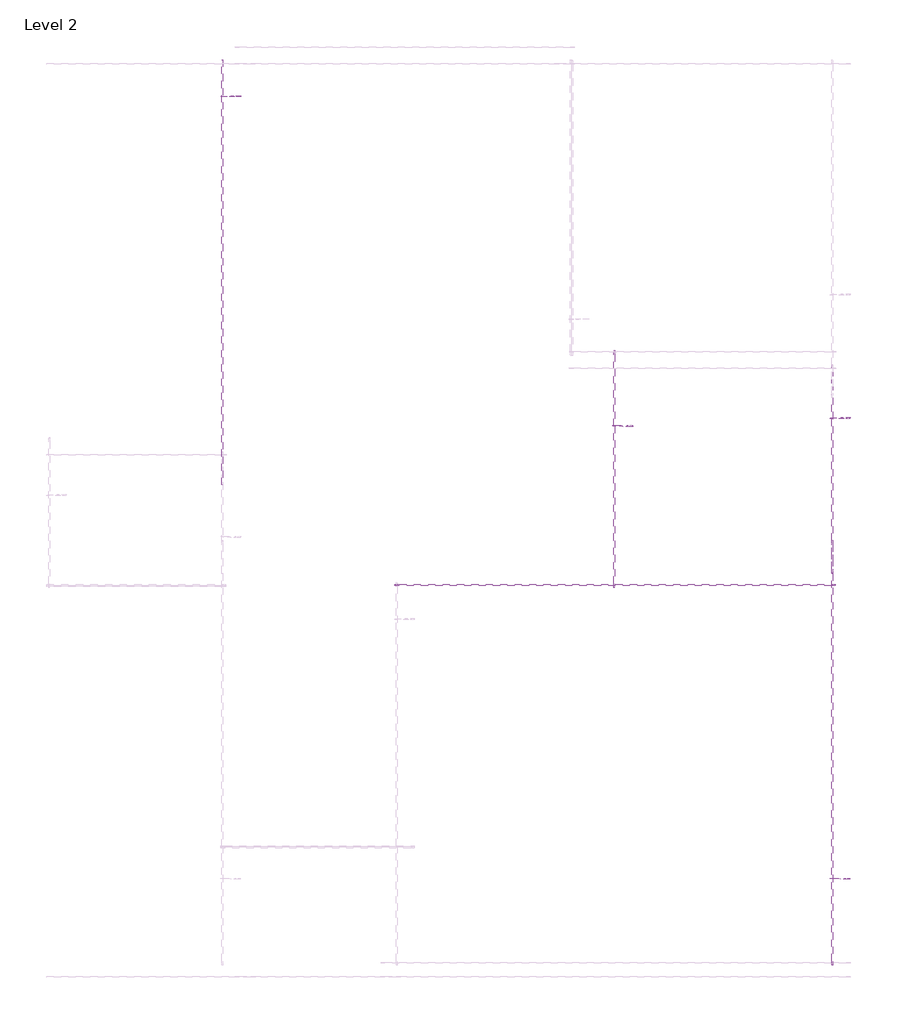
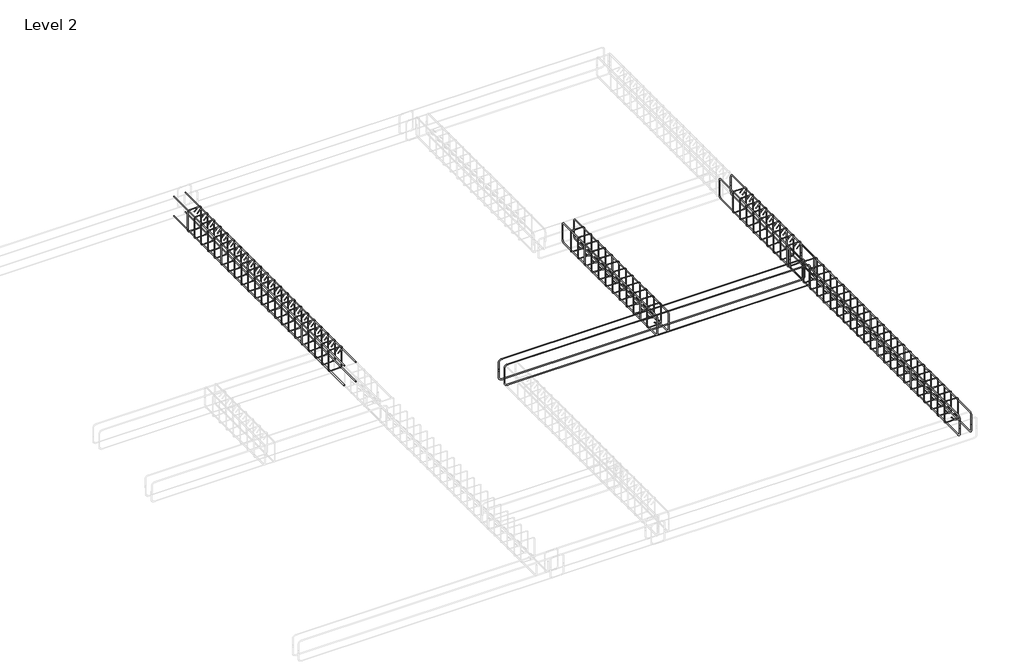
# One storey, part 4 of 5: 14 reinforcing bars.
"""IFC4 building model written with IfcOpenShell, lengths in millimetres."""

from ifc_helpers import new_model, si_unit, point, frame, origin, place, context, project, spatial, polyline, circle_curve, trimmed, segment, composite_curve, source, transform, mapped, element, save
from ifc_brep_helpers import swept_disk

model = new_model("IFC4")

# Units and contexts
model_context = context("Model", 3, world=origin())
ifc_project = project(units=[si_unit("LENGTHUNIT", "METRE", prefix="MILLI")], contexts=[model_context])

# Site, building, storey
site = spatial("IfcSite", under=ifc_project)
building = spatial("IfcBuilding", under=site)
storey = spatial("IfcBuildingStorey", under=building, Name="Level 2", Elevation=3048.0)

# Reinforcing bars
placement = place(None, origin())
reinforcing_bar_shape = source(origin(), model_context, "Body", "SolidModel", [
    swept_disk(composite_curve([segment(polyline([(-4212.455746, 4821.0577522, 5841.8967919), (-4212.455746, 4821.0577522, 5994.2967919)]), True, "CONTINUOUS"), segment(trimmed(circle_curve(frame((-4212.455746, 4776.9887522, 5994.2967919), z_axis=(1.0, 0.0, 0.0), x_axis=(0.0, 44.069000000000415, 0.0)), 44.069), [point((-4212.455746, 4821.0577522, 5994.2967919))], [point((-4212.455746, 4776.9887522, 6038.3657919))], True, "CARTESIAN"), True, "CONTINUOUS"), segment(polyline([(-4212.455746, 4776.9887522, 6038.3657919), (-4212.455746, 2478.6647522, 6038.3657919)]), True, "CONTINUOUS"), segment(trimmed(circle_curve(frame((-4212.455746, 2478.6647522, 5994.2967919), z_axis=(1.0, 0.0, 0.0), x_axis=(0.0, 0.0, 44.068999999999505)), 44.069), [point((-4212.455746, 2478.6647522, 6038.3657919))], [point((-4212.455746, 2434.5957522, 5994.2967919))], True, "CARTESIAN"), True, "CONTINUOUS"), segment(polyline([(-4212.455746, 2434.5957522, 5994.2967919), (-4212.455746, 2434.5957522, 5841.8967919)]), True, "CONTINUOUS")], self_intersect=False), 5.969),
])
element("IfcReinforcingBar", 1, at=placement, inside=storey, context=model_context, shape_type="MappedRepresentation", body=[
    mapped(reinforcing_bar_shape, transform((0.0, 0.0, 0.0), x_axis=(1.0, 0.0, 0.0), y_axis=(0.0, 1.0, 0.0), z_axis=(0.0, 0.0, 1.0))),
    mapped(reinforcing_bar_shape, transform((-189.5315837, 0.0, 0.0), x_axis=(1.0, 0.0, 0.0), y_axis=(0.0, 1.0, 0.0), z_axis=(0.0, 0.0, 1.0))),
])
reinforcing_bar_2_shape = source(origin(), model_context, "Body", "SolidModel", [
    swept_disk(composite_curve([segment(polyline([(-4212.455746, 2434.5957522, 5892.9032081), (-4212.455746, 2434.5957522, 5740.5032081)]), True, "CONTINUOUS"), segment(trimmed(circle_curve(frame((-4212.455746, 2478.6647522, 5740.5032081), z_axis=(1.0, 0.0, 0.0), x_axis=(0.0, -44.06899999999996, 0.0)), 44.069), [point((-4212.455746, 2434.5957522, 5740.5032081))], [point((-4212.455746, 2478.6647522, 5696.4342081))], True, "CARTESIAN"), True, "CONTINUOUS"), segment(polyline([(-4212.455746, 2478.6647522, 5696.4342081), (-4212.455746, 4776.9887522, 5696.4342081)]), True, "CONTINUOUS"), segment(trimmed(circle_curve(frame((-4212.455746, 4776.9887522, 5740.5032081), z_axis=(1.0, 0.0, 0.0), x_axis=(0.0, 0.0, -44.068999999999505)), 44.069), [point((-4212.455746, 4776.9887522, 5696.4342081))], [point((-4212.455746, 4821.0577522, 5740.5032081))], True, "CARTESIAN"), True, "CONTINUOUS"), segment(polyline([(-4212.455746, 4821.0577522, 5740.5032081), (-4212.455746, 4821.0577522, 5892.9032081)]), True, "CONTINUOUS")], self_intersect=False), 5.969),
])
element("IfcReinforcingBar", 2, at=placement, inside=storey, context=model_context, shape_type="MappedRepresentation", body=[
    mapped(reinforcing_bar_2_shape, transform((0.0, 0.0, 0.0), x_axis=(1.0, 0.0, 0.0), y_axis=(0.0, 1.0, 0.0), z_axis=(0.0, 0.0, 1.0))),
    mapped(reinforcing_bar_2_shape, transform((-189.5315837, 0.0, 0.0), x_axis=(1.0, 0.0, 0.0), y_axis=(0.0, 1.0, 0.0), z_axis=(0.0, 0.0, 1.0))),
])
reinforcing_bar_3_shape = source(origin(), model_context, "Body", "SolidModel", [
    swept_disk(composite_curve([segment(polyline([(-4212.455746, 2803.6577522, 5841.8967919), (-4212.455746, 2803.6577522, 5994.2967919)]), True, "CONTINUOUS"), segment(trimmed(circle_curve(frame((-4212.455746, 2759.5887522, 5994.2967919), z_axis=(1.0, 0.0, 0.0), x_axis=(0.0, 44.06899999999996, 0.0)), 44.069), [point((-4212.455746, 2803.6577522, 5994.2967919))], [point((-4212.455746, 2759.5887522, 6038.3657919))], True, "CARTESIAN"), True, "CONTINUOUS"), segment(polyline([(-4212.455746, 2759.5887522, 6038.3657919), (-4212.455746, -2021.3352478, 6038.3657919)]), True, "CONTINUOUS"), segment(trimmed(circle_curve(frame((-4212.455746, -2021.3352478, 5994.2967919), z_axis=(1.0, 0.0, 0.0), x_axis=(0.0, 0.0, 44.068999999999505)), 44.069), [point((-4212.455746, -2021.3352478, 6038.3657919))], [point((-4212.455746, -2065.4042478, 5994.2967919))], True, "CARTESIAN"), True, "CONTINUOUS"), segment(polyline([(-4212.455746, -2065.4042478, 5994.2967919), (-4212.455746, -2065.4042478, 5841.8967919)]), True, "CONTINUOUS")], self_intersect=False), 5.969),
])
element("IfcReinforcingBar", 3, at=placement, inside=storey, context=model_context, shape_type="MappedRepresentation", body=[
    mapped(reinforcing_bar_3_shape, transform((0.0, 0.0, 0.0), x_axis=(1.0, 0.0, 0.0), y_axis=(0.0, 1.0, 0.0), z_axis=(0.0, 0.0, 1.0))),
    mapped(reinforcing_bar_3_shape, transform((-189.5315837, 0.0, 0.0), x_axis=(1.0, 0.0, 0.0), y_axis=(0.0, 1.0, 0.0), z_axis=(0.0, 0.0, 1.0))),
])
reinforcing_bar_4_shape = source(origin(), model_context, "Body", "SolidModel", [
    swept_disk(composite_curve([segment(polyline([(-4212.455746, -2065.4042478, 5892.9032081), (-4212.455746, -2065.4042478, 5740.5032081)]), True, "CONTINUOUS"), segment(trimmed(circle_curve(frame((-4212.455746, -2021.3352478, 5740.5032081), z_axis=(1.0, 0.0, 0.0), x_axis=(0.0, -44.06900000000019, 0.0)), 44.069), [point((-4212.455746, -2065.4042478, 5740.5032081))], [point((-4212.455746, -2021.3352478, 5696.4342081))], True, "CARTESIAN"), True, "CONTINUOUS"), segment(polyline([(-4212.455746, -2021.3352478, 5696.4342081), (-4212.455746, 2759.5887522, 5696.4342081)]), True, "CONTINUOUS"), segment(trimmed(circle_curve(frame((-4212.455746, 2759.5887522, 5740.5032081), z_axis=(1.0, 0.0, 0.0), x_axis=(0.0, 0.0, -44.068999999999505)), 44.069), [point((-4212.455746, 2759.5887522, 5696.4342081))], [point((-4212.455746, 2803.6577522, 5740.5032081))], True, "CARTESIAN"), True, "CONTINUOUS"), segment(polyline([(-4212.455746, 2803.6577522, 5740.5032081), (-4212.455746, 2803.6577522, 5892.9032081)]), True, "CONTINUOUS")], self_intersect=False), 5.969),
])
element("IfcReinforcingBar", 4, at=placement, inside=storey, context=model_context, shape_type="MappedRepresentation", body=[
    mapped(reinforcing_bar_4_shape, transform((0.0, 0.0, 0.0), x_axis=(1.0, 0.0, 0.0), y_axis=(0.0, 1.0, 0.0), z_axis=(0.0, 0.0, 1.0))),
    mapped(reinforcing_bar_4_shape, transform((-189.5315837, 0.0, 0.0), x_axis=(1.0, 0.0, 0.0), y_axis=(0.0, 1.0, 0.0), z_axis=(0.0, 0.0, 1.0))),
])
reinforcing_bar_5_shape = source(origin(), model_context, "Body", "SolidModel", [
    swept_disk(composite_curve([segment(polyline([(-4260.3161447, -1648.3362478, 5785.7833901), (-4205.4511463, -1648.3362478, 5730.9183916)]), True, "CONTINUOUS"), segment(trimmed(circle_curve(frame((-4226.1955379, -1648.3362478, 5710.174), z_axis=(0.0, 1.0, 0.0), x_axis=(20.7443916000002, 0.0, 20.7443916000002)), 29.337), [point((-4205.4511463, -1648.3362478, 5730.9183916))], [point((-4226.1955379, -1648.3362478, 5680.837))], True, "CARTESIAN"), True, "CONTINUOUS"), segment(polyline([(-4226.1955379, -1648.3362478, 5680.837), (-4388.2475379, -1648.3362478, 5680.837)]), True, "CONTINUOUS"), segment(trimmed(circle_curve(frame((-4388.2475379, -1648.3362478, 5710.174), z_axis=(0.0, 1.0, 0.0), x_axis=(0.0, 0.0, -29.336999999999534)), 29.337), [point((-4388.2475379, -1648.3362478, 5680.837))], [point((-4417.5845379, -1648.3362478, 5710.174))], True, "CARTESIAN"), True, "CONTINUOUS"), segment(polyline([(-4417.5845379, -1648.3362478, 5710.174), (-4417.5845379, -1648.3362478, 6024.626)]), True, "CONTINUOUS"), segment(trimmed(circle_curve(frame((-4388.2661869, -1649.3821269, 6024.626), z_axis=(0.03565051078635361, 0.9993643184948481, 0.0), x_axis=(-29.318350999999893, 1.0458791000000929, 0.0)), 29.337), [point((-4417.5845379, -1648.3362478, 6024.626))], [point((-4388.2661869, -1649.3821269, 6053.963))], True, "CARTESIAN"), True, "CONTINUOUS"), segment(polyline([(-4388.2661869, -1649.3821269, 6053.963), (-4226.1768889, -1655.1643688, 6053.963)]), True, "CONTINUOUS"), segment(trimmed(circle_curve(frame((-4226.1768889, -1655.1643688, 6024.626), z_axis=(0.03565051078635361, 0.9993643184948481, 0.0), x_axis=(0.0, 0.0, 29.336999999999534)), 29.337), [point((-4226.1768889, -1655.1643688, 6053.963))], [point((-4196.8585379, -1656.2102478, 6024.626))], True, "CARTESIAN"), True, "CONTINUOUS"), segment(polyline([(-4196.8585379, -1656.2102478, 6024.626), (-4196.8585379, -1656.2102478, 5710.174)]), True, "CONTINUOUS"), segment(trimmed(circle_curve(frame((-4226.1955379, -1656.2102478, 5710.174), z_axis=(0.0, 1.0, 0.0), x_axis=(29.337000000000444, 0.0, 0.0)), 29.337), [point((-4196.8585379, -1656.2102478, 5710.174))], [point((-4246.9399295, -1656.2102478, 5689.4296084))], True, "CARTESIAN"), True, "CONTINUOUS"), segment(polyline([(-4246.9399295, -1656.2102478, 5689.4296084), (-4301.804928, -1656.2102478, 5744.2946068)]), True, "CONTINUOUS")], self_intersect=False), 3.937),
])
element("IfcReinforcingBar", 5, at=placement, inside=storey, context=model_context, shape_type="MappedRepresentation", body=[
    mapped(reinforcing_bar_5_shape, transform((0.0, 0.0, 0.0), x_axis=(1.0, 0.0, 0.0), y_axis=(0.0, 1.0, 0.0), z_axis=(0.0, 0.0, 1.0))),
    mapped(reinforcing_bar_5_shape, transform((0.0, 192.1393333, 0.0), x_axis=(1.0, 0.0, 0.0), y_axis=(0.0, 1.0, 0.0), z_axis=(0.0, 0.0, 1.0))),
    mapped(reinforcing_bar_5_shape, transform((0.0, 384.2786667, 0.0), x_axis=(1.0, 0.0, 0.0), y_axis=(0.0, 1.0, 0.0), z_axis=(0.0, 0.0, 1.0))),
    mapped(reinforcing_bar_5_shape, transform((0.0, 576.418, 0.0), x_axis=(1.0, 0.0, 0.0), y_axis=(0.0, 1.0, 0.0), z_axis=(0.0, 0.0, 1.0))),
    mapped(reinforcing_bar_5_shape, transform((0.0, 768.5573333, 0.0), x_axis=(1.0, 0.0, 0.0), y_axis=(0.0, 1.0, 0.0), z_axis=(0.0, 0.0, 1.0))),
    mapped(reinforcing_bar_5_shape, transform((0.0, 960.6966667, 0.0), x_axis=(1.0, 0.0, 0.0), y_axis=(0.0, 1.0, 0.0), z_axis=(0.0, 0.0, 1.0))),
    mapped(reinforcing_bar_5_shape, transform((0.0, 1152.836, 0.0), x_axis=(1.0, 0.0, 0.0), y_axis=(0.0, 1.0, 0.0), z_axis=(0.0, 0.0, 1.0))),
    mapped(reinforcing_bar_5_shape, transform((0.0, 1344.9753333, 0.0), x_axis=(1.0, 0.0, 0.0), y_axis=(0.0, 1.0, 0.0), z_axis=(0.0, 0.0, 1.0))),
    mapped(reinforcing_bar_5_shape, transform((0.0, 1537.1146667, 0.0), x_axis=(1.0, 0.0, 0.0), y_axis=(0.0, 1.0, 0.0), z_axis=(0.0, 0.0, 1.0))),
    mapped(reinforcing_bar_5_shape, transform((0.0, 1729.254, 0.0), x_axis=(1.0, 0.0, 0.0), y_axis=(0.0, 1.0, 0.0), z_axis=(0.0, 0.0, 1.0))),
    mapped(reinforcing_bar_5_shape, transform((0.0, 1921.3933333, 0.0), x_axis=(1.0, 0.0, 0.0), y_axis=(0.0, 1.0, 0.0), z_axis=(0.0, 0.0, 1.0))),
    mapped(reinforcing_bar_5_shape, transform((0.0, 2113.5326667, 0.0), x_axis=(1.0, 0.0, 0.0), y_axis=(0.0, 1.0, 0.0), z_axis=(0.0, 0.0, 1.0))),
    mapped(reinforcing_bar_5_shape, transform((0.0, 2305.672, 0.0), x_axis=(1.0, 0.0, 0.0), y_axis=(0.0, 1.0, 0.0), z_axis=(0.0, 0.0, 1.0))),
    mapped(reinforcing_bar_5_shape, transform((0.0, 2497.8113333, 0.0), x_axis=(1.0, 0.0, 0.0), y_axis=(0.0, 1.0, 0.0), z_axis=(0.0, 0.0, 1.0))),
    mapped(reinforcing_bar_5_shape, transform((0.0, 2689.9506667, 0.0), x_axis=(1.0, 0.0, 0.0), y_axis=(0.0, 1.0, 0.0), z_axis=(0.0, 0.0, 1.0))),
    mapped(reinforcing_bar_5_shape, transform((0.0, 2882.09, 0.0), x_axis=(1.0, 0.0, 0.0), y_axis=(0.0, 1.0, 0.0), z_axis=(0.0, 0.0, 1.0))),
    mapped(reinforcing_bar_5_shape, transform((0.0, 3074.2293333, 0.0), x_axis=(1.0, 0.0, 0.0), y_axis=(0.0, 1.0, 0.0), z_axis=(0.0, 0.0, 1.0))),
    mapped(reinforcing_bar_5_shape, transform((0.0, 3266.3686667, 0.0), x_axis=(1.0, 0.0, 0.0), y_axis=(0.0, 1.0, 0.0), z_axis=(0.0, 0.0, 1.0))),
    mapped(reinforcing_bar_5_shape, transform((0.0, 3458.508, 0.0), x_axis=(1.0, 0.0, 0.0), y_axis=(0.0, 1.0, 0.0), z_axis=(0.0, 0.0, 1.0))),
    mapped(reinforcing_bar_5_shape, transform((0.0, 3650.6473333, 0.0), x_axis=(1.0, 0.0, 0.0), y_axis=(0.0, 1.0, 0.0), z_axis=(0.0, 0.0, 1.0))),
    mapped(reinforcing_bar_5_shape, transform((0.0, 3842.7866667, 0.0), x_axis=(1.0, 0.0, 0.0), y_axis=(0.0, 1.0, 0.0), z_axis=(0.0, 0.0, 1.0))),
    mapped(reinforcing_bar_5_shape, transform((0.0, 4034.926, 0.0), x_axis=(1.0, 0.0, 0.0), y_axis=(0.0, 1.0, 0.0), z_axis=(0.0, 0.0, 1.0))),
])
reinforcing_bar_6_shape = source(origin(), model_context, "Body", "SolidModel", [
    swept_disk(composite_curve([segment(polyline([(-4260.3161447, 4403.9897522, 5949.0166099), (-4205.4511463, 4403.9897522, 6003.8816084)]), True, "CONTINUOUS"), segment(trimmed(circle_curve(frame((-4226.1955379, 4403.9897522, 6024.626), z_axis=(0.0, -1.0, 0.0), x_axis=(20.7443916000002, 0.0, -20.7443916000002)), 29.337), [point((-4205.4511463, 4403.9897522, 6003.8816084))], [point((-4226.1955379, 4403.9897522, 6053.963))], True, "CARTESIAN"), True, "CONTINUOUS"), segment(polyline([(-4226.1955379, 4403.9897522, 6053.963), (-4388.2475379, 4403.9897522, 6053.963)]), True, "CONTINUOUS"), segment(trimmed(circle_curve(frame((-4388.2475379, 4403.9897522, 6024.626), z_axis=(0.0, -1.0, 0.0), x_axis=(0.0, 0.0, 29.336999999999534)), 29.337), [point((-4388.2475379, 4403.9897522, 6053.963))], [point((-4417.5845379, 4403.9897522, 6024.626))], True, "CARTESIAN"), True, "CONTINUOUS"), segment(polyline([(-4417.5845379, 4403.9897522, 6024.626), (-4417.5845379, 4403.9897522, 5710.174)]), True, "CONTINUOUS"), segment(trimmed(circle_curve(frame((-4388.2661869, 4405.0356312, 5710.174), z_axis=(0.03565051078635044, -0.9993643184948482, 0.0), x_axis=(-29.318350999999893, -1.045879000000241, 0.0)), 29.337), [point((-4417.5845379, 4403.9897522, 5710.174))], [point((-4388.2661869, 4405.0356312, 5680.837))], True, "CARTESIAN"), True, "CONTINUOUS"), segment(polyline([(-4388.2661869, 4405.0356312, 5680.837), (-4226.1768889, 4410.8178731, 5680.837)]), True, "CONTINUOUS"), segment(trimmed(circle_curve(frame((-4226.1768889, 4410.8178731, 5710.174), z_axis=(0.03565051078635044, -0.9993643184948482, 0.0), x_axis=(0.0, 0.0, -29.336999999999534)), 29.337), [point((-4226.1768889, 4410.8178731, 5680.837))], [point((-4196.8585379, 4411.8637522, 5710.174))], True, "CARTESIAN"), True, "CONTINUOUS"), segment(polyline([(-4196.8585379, 4411.8637522, 5710.174), (-4196.8585379, 4411.8637522, 6024.626)]), True, "CONTINUOUS"), segment(trimmed(circle_curve(frame((-4226.1955379, 4411.8637522, 6024.626), z_axis=(0.0, -1.0, 0.0), x_axis=(29.337000000000444, 0.0, 0.0)), 29.337), [point((-4196.8585379, 4411.8637522, 6024.626))], [point((-4246.9399295, 4411.8637522, 6045.3703916))], True, "CARTESIAN"), True, "CONTINUOUS"), segment(polyline([(-4246.9399295, 4411.8637522, 6045.3703916), (-4301.804928, 4411.8637522, 5990.5053932)]), True, "CONTINUOUS")], self_intersect=False), 3.937),
])
element("IfcReinforcingBar", 6, at=placement, inside=storey, context=model_context, shape_type="MappedRepresentation", body=[
    mapped(reinforcing_bar_6_shape, transform((0.0, 0.0, 0.0), x_axis=(1.0, 0.0, 0.0), y_axis=(0.0, 1.0, 0.0), z_axis=(0.0, 0.0, 1.0))),
    mapped(reinforcing_bar_6_shape, transform((0.0, -194.04075, 0.0), x_axis=(1.0, 0.0, 0.0), y_axis=(0.0, 1.0, 0.0), z_axis=(0.0, 0.0, 1.0))),
    mapped(reinforcing_bar_6_shape, transform((0.0, -388.0815, 0.0), x_axis=(1.0, 0.0, 0.0), y_axis=(0.0, 1.0, 0.0), z_axis=(0.0, 0.0, 1.0))),
    mapped(reinforcing_bar_6_shape, transform((0.0, -582.12225, 0.0), x_axis=(1.0, 0.0, 0.0), y_axis=(0.0, 1.0, 0.0), z_axis=(0.0, 0.0, 1.0))),
    mapped(reinforcing_bar_6_shape, transform((0.0, -776.163, 0.0), x_axis=(1.0, 0.0, 0.0), y_axis=(0.0, 1.0, 0.0), z_axis=(0.0, 0.0, 1.0))),
    mapped(reinforcing_bar_6_shape, transform((0.0, -970.20375, 0.0), x_axis=(1.0, 0.0, 0.0), y_axis=(0.0, 1.0, 0.0), z_axis=(0.0, 0.0, 1.0))),
    mapped(reinforcing_bar_6_shape, transform((0.0, -1164.2445, 0.0), x_axis=(1.0, 0.0, 0.0), y_axis=(0.0, 1.0, 0.0), z_axis=(0.0, 0.0, 1.0))),
    mapped(reinforcing_bar_6_shape, transform((0.0, -1358.28525, 0.0), x_axis=(1.0, 0.0, 0.0), y_axis=(0.0, 1.0, 0.0), z_axis=(0.0, 0.0, 1.0))),
    mapped(reinforcing_bar_6_shape, transform((0.0, -1552.326, 0.0), x_axis=(1.0, 0.0, 0.0), y_axis=(0.0, 1.0, 0.0), z_axis=(0.0, 0.0, 1.0))),
])
reinforcing_bar_7_shape = source(origin(), model_context, "Body", "SolidModel", [
    swept_disk(composite_curve([segment(polyline([(-11212.455746, 8327.0267522, 6038.3657919), (-11212.455746, 3446.0267522, 6038.3657919)]), True, "CONTINUOUS")], self_intersect=False), 5.969),
])
element("IfcReinforcingBar", 7, at=placement, inside=storey, context=model_context, shape_type="MappedRepresentation", body=[
    mapped(reinforcing_bar_7_shape, transform((0.0, 0.0, 0.0), x_axis=(1.0, 0.0, 0.0), y_axis=(0.0, 1.0, 0.0), z_axis=(0.0, 0.0, 1.0))),
    mapped(reinforcing_bar_7_shape, transform((-189.5315837, 0.0, 0.0), x_axis=(1.0, 0.0, 0.0), y_axis=(0.0, 1.0, 0.0), z_axis=(0.0, 0.0, 1.0))),
])
reinforcing_bar_8_shape = source(origin(), model_context, "Body", "SolidModel", [
    swept_disk(composite_curve([segment(polyline([(-11212.455746, 3446.0267522, 5696.4342081), (-11212.455746, 8327.0267522, 5696.4342081)]), True, "CONTINUOUS")], self_intersect=False), 5.969),
])
element("IfcReinforcingBar", 8, at=placement, inside=storey, context=model_context, shape_type="MappedRepresentation", body=[
    mapped(reinforcing_bar_8_shape, transform((0.0, 0.0, 0.0), x_axis=(1.0, 0.0, 0.0), y_axis=(0.0, 1.0, 0.0), z_axis=(0.0, 0.0, 1.0))),
    mapped(reinforcing_bar_8_shape, transform((-189.5315837, 0.0, 0.0), x_axis=(1.0, 0.0, 0.0), y_axis=(0.0, 1.0, 0.0), z_axis=(0.0, 0.0, 1.0))),
])
reinforcing_bar_9_shape = source(origin(), model_context, "Body", "SolidModel", [
    swept_disk(composite_curve([segment(polyline([(-11260.3161447, 7903.9897522, 5949.0166099), (-11205.4511463, 7903.9897522, 6003.8816084)]), True, "CONTINUOUS"), segment(trimmed(circle_curve(frame((-11226.1955379, 7903.9897522, 6024.626), z_axis=(0.0, -1.0, 0.0), x_axis=(20.74439159999929, 0.0, -20.7443916000002)), 29.337), [point((-11205.4511463, 7903.9897522, 6003.8816084))], [point((-11226.1955379, 7903.9897522, 6053.963))], True, "CARTESIAN"), True, "CONTINUOUS"), segment(polyline([(-11226.1955379, 7903.9897522, 6053.963), (-11388.2475379, 7903.9897522, 6053.963)]), True, "CONTINUOUS"), segment(trimmed(circle_curve(frame((-11388.2475379, 7903.9897522, 6024.626), z_axis=(0.0, -1.0, 0.0), x_axis=(0.0, 0.0, 29.336999999999534)), 29.337), [point((-11388.2475379, 7903.9897522, 6053.963))], [point((-11417.5845379, 7903.9897522, 6024.626))], True, "CARTESIAN"), True, "CONTINUOUS"), segment(polyline([(-11417.5845379, 7903.9897522, 6024.626), (-11417.5845379, 7903.9897522, 5710.174)]), True, "CONTINUOUS"), segment(trimmed(circle_curve(frame((-11388.2661869, 7905.0356312, 5710.174), z_axis=(0.035650510786351154, -0.9993643184948482, 0.0), x_axis=(-29.318350999999893, -1.045879000000241, 0.0)), 29.337), [point((-11417.5845379, 7903.9897522, 5710.174))], [point((-11388.2661869, 7905.0356312, 5680.837))], True, "CARTESIAN"), True, "CONTINUOUS"), segment(polyline([(-11388.2661869, 7905.0356312, 5680.837), (-11226.1768889, 7910.8178731, 5680.837)]), True, "CONTINUOUS"), segment(trimmed(circle_curve(frame((-11226.1768889, 7910.8178731, 5710.174), z_axis=(0.035650510786351154, -0.9993643184948482, 0.0), x_axis=(0.0, 0.0, -29.336999999999534)), 29.337), [point((-11226.1768889, 7910.8178731, 5680.837))], [point((-11196.8585379, 7911.8637522, 5710.174))], True, "CARTESIAN"), True, "CONTINUOUS"), segment(polyline([(-11196.8585379, 7911.8637522, 5710.174), (-11196.8585379, 7911.8637522, 6024.626)]), True, "CONTINUOUS"), segment(trimmed(circle_curve(frame((-11226.1955379, 7911.8637522, 6024.626), z_axis=(0.0, -1.0, 0.0), x_axis=(29.336999999999534, 0.0, 0.0)), 29.337), [point((-11196.8585379, 7911.8637522, 6024.626))], [point((-11246.9399295, 7911.8637522, 6045.3703916))], True, "CARTESIAN"), True, "CONTINUOUS"), segment(polyline([(-11246.9399295, 7911.8637522, 6045.3703916), (-11301.804928, 7911.8637522, 5990.5053932)]), True, "CONTINUOUS")], self_intersect=False), 3.937),
])
element("IfcReinforcingBar", 9, at=placement, inside=storey, context=model_context, shape_type="MappedRepresentation", body=[
    mapped(reinforcing_bar_9_shape, transform((0.0, 0.0, 0.0), x_axis=(1.0, 0.0, 0.0), y_axis=(0.0, 1.0, 0.0), z_axis=(0.0, 0.0, 1.0))),
    mapped(reinforcing_bar_9_shape, transform((0.0, -192.1393333, 0.0), x_axis=(1.0, 0.0, 0.0), y_axis=(0.0, 1.0, 0.0), z_axis=(0.0, 0.0, 1.0))),
    mapped(reinforcing_bar_9_shape, transform((0.0, -384.2786667, 0.0), x_axis=(1.0, 0.0, 0.0), y_axis=(0.0, 1.0, 0.0), z_axis=(0.0, 0.0, 1.0))),
    mapped(reinforcing_bar_9_shape, transform((0.0, -576.418, 0.0), x_axis=(1.0, 0.0, 0.0), y_axis=(0.0, 1.0, 0.0), z_axis=(0.0, 0.0, 1.0))),
    mapped(reinforcing_bar_9_shape, transform((0.0, -768.5573333, 0.0), x_axis=(1.0, 0.0, 0.0), y_axis=(0.0, 1.0, 0.0), z_axis=(0.0, 0.0, 1.0))),
    mapped(reinforcing_bar_9_shape, transform((0.0, -960.6966667, 0.0), x_axis=(1.0, 0.0, 0.0), y_axis=(0.0, 1.0, 0.0), z_axis=(0.0, 0.0, 1.0))),
    mapped(reinforcing_bar_9_shape, transform((0.0, -1152.836, 0.0), x_axis=(1.0, 0.0, 0.0), y_axis=(0.0, 1.0, 0.0), z_axis=(0.0, 0.0, 1.0))),
    mapped(reinforcing_bar_9_shape, transform((0.0, -1344.9753333, 0.0), x_axis=(1.0, 0.0, 0.0), y_axis=(0.0, 1.0, 0.0), z_axis=(0.0, 0.0, 1.0))),
    mapped(reinforcing_bar_9_shape, transform((0.0, -1537.1146667, 0.0), x_axis=(1.0, 0.0, 0.0), y_axis=(0.0, 1.0, 0.0), z_axis=(0.0, 0.0, 1.0))),
    mapped(reinforcing_bar_9_shape, transform((0.0, -1729.254, 0.0), x_axis=(1.0, 0.0, 0.0), y_axis=(0.0, 1.0, 0.0), z_axis=(0.0, 0.0, 1.0))),
    mapped(reinforcing_bar_9_shape, transform((0.0, -1921.3933333, 0.0), x_axis=(1.0, 0.0, 0.0), y_axis=(0.0, 1.0, 0.0), z_axis=(0.0, 0.0, 1.0))),
    mapped(reinforcing_bar_9_shape, transform((0.0, -2113.5326667, 0.0), x_axis=(1.0, 0.0, 0.0), y_axis=(0.0, 1.0, 0.0), z_axis=(0.0, 0.0, 1.0))),
    mapped(reinforcing_bar_9_shape, transform((0.0, -2305.672, 0.0), x_axis=(1.0, 0.0, 0.0), y_axis=(0.0, 1.0, 0.0), z_axis=(0.0, 0.0, 1.0))),
    mapped(reinforcing_bar_9_shape, transform((0.0, -2497.8113333, 0.0), x_axis=(1.0, 0.0, 0.0), y_axis=(0.0, 1.0, 0.0), z_axis=(0.0, 0.0, 1.0))),
    mapped(reinforcing_bar_9_shape, transform((0.0, -2689.9506667, 0.0), x_axis=(1.0, 0.0, 0.0), y_axis=(0.0, 1.0, 0.0), z_axis=(0.0, 0.0, 1.0))),
    mapped(reinforcing_bar_9_shape, transform((0.0, -2882.09, 0.0), x_axis=(1.0, 0.0, 0.0), y_axis=(0.0, 1.0, 0.0), z_axis=(0.0, 0.0, 1.0))),
    mapped(reinforcing_bar_9_shape, transform((0.0, -3074.2293333, 0.0), x_axis=(1.0, 0.0, 0.0), y_axis=(0.0, 1.0, 0.0), z_axis=(0.0, 0.0, 1.0))),
    mapped(reinforcing_bar_9_shape, transform((0.0, -3266.3686667, 0.0), x_axis=(1.0, 0.0, 0.0), y_axis=(0.0, 1.0, 0.0), z_axis=(0.0, 0.0, 1.0))),
    mapped(reinforcing_bar_9_shape, transform((0.0, -3458.508, 0.0), x_axis=(1.0, 0.0, 0.0), y_axis=(0.0, 1.0, 0.0), z_axis=(0.0, 0.0, 1.0))),
    mapped(reinforcing_bar_9_shape, transform((0.0, -3650.6473333, 0.0), x_axis=(1.0, 0.0, 0.0), y_axis=(0.0, 1.0, 0.0), z_axis=(0.0, 0.0, 1.0))),
    mapped(reinforcing_bar_9_shape, transform((0.0, -3842.7866667, 0.0), x_axis=(1.0, 0.0, 0.0), y_axis=(0.0, 1.0, 0.0), z_axis=(0.0, 0.0, 1.0))),
    mapped(reinforcing_bar_9_shape, transform((0.0, -4034.926, 0.0), x_axis=(1.0, 0.0, 0.0), y_axis=(0.0, 1.0, 0.0), z_axis=(0.0, 0.0, 1.0))),
])
reinforcing_bar_10_shape = source(origin(), model_context, "Body", "SolidModel", [
    swept_disk(composite_curve([segment(polyline([(-4363.9905379, 2458.8527522, 5847.588), (-4363.9905379, 2458.8527522, 5999.988)]), True, "CONTINUOUS"), segment(trimmed(circle_curve(frame((-4408.0595379, 2458.8527522, 5999.988), z_axis=(0.0, -1.0, 0.0), x_axis=(44.068999999999505, 0.0, 0.0)), 44.069), [point((-4363.9905379, 2458.8527522, 5999.988))], [point((-4408.0595379, 2458.8527522, 6044.057))], True, "CARTESIAN"), True, "CONTINUOUS"), segment(polyline([(-4408.0595379, 2458.8527522, 6044.057), (-9371.4835379, 2458.8527522, 6044.057)]), True, "CONTINUOUS"), segment(trimmed(circle_curve(frame((-9371.4835379, 2458.8527522, 5999.988), z_axis=(0.0, -1.0, 0.0), x_axis=(0.0, 0.0, 44.068999999999505)), 44.069), [point((-9371.4835379, 2458.8527522, 6044.057))], [point((-9415.5525379, 2458.8527522, 5999.988))], True, "CARTESIAN"), True, "CONTINUOUS"), segment(polyline([(-9415.5525379, 2458.8527522, 5999.988), (-9415.5525379, 2458.8527522, 5847.588)]), True, "CONTINUOUS")], self_intersect=False), 5.969),
])
element("IfcReinforcingBar", 10, at=placement, inside=storey, context=model_context, shape_type="MappedRepresentation", body=[
    mapped(reinforcing_bar_10_shape, transform((0.0, 0.0, 0.0), x_axis=(1.0, 0.0, 0.0), y_axis=(0.0, 1.0, 0.0), z_axis=(0.0, 0.0, 1.0))),
    mapped(reinforcing_bar_10_shape, transform((0.0, -162.052, 0.0), x_axis=(1.0, 0.0, 0.0), y_axis=(0.0, 1.0, 0.0), z_axis=(0.0, 0.0, 1.0))),
])
reinforcing_bar_11_shape = source(origin(), model_context, "Body", "SolidModel", [
    swept_disk(composite_curve([segment(polyline([(-9415.5525379, 2296.8007522, 5887.212), (-9415.5525379, 2296.8007522, 5734.812)]), True, "CONTINUOUS"), segment(trimmed(circle_curve(frame((-9371.4835379, 2296.8007522, 5734.812), z_axis=(0.0, -1.0, 0.0), x_axis=(-44.068999999999505, 0.0, 0.0)), 44.069), [point((-9415.5525379, 2296.8007522, 5734.812))], [point((-9371.4835379, 2296.8007522, 5690.743))], True, "CARTESIAN"), True, "CONTINUOUS"), segment(polyline([(-9371.4835379, 2296.8007522, 5690.743), (-4408.0595379, 2296.8007522, 5690.743)]), True, "CONTINUOUS"), segment(trimmed(circle_curve(frame((-4408.0595379, 2296.8007522, 5734.812), z_axis=(0.0, -1.0, 0.0), x_axis=(0.0, 0.0, -44.068999999999505)), 44.069), [point((-4408.0595379, 2296.8007522, 5690.743))], [point((-4363.9905379, 2296.8007522, 5734.812))], True, "CARTESIAN"), True, "CONTINUOUS"), segment(polyline([(-4363.9905379, 2296.8007522, 5734.812), (-4363.9905379, 2296.8007522, 5887.212)]), True, "CONTINUOUS")], self_intersect=False), 5.969),
])
element("IfcReinforcingBar", 11, at=placement, inside=storey, context=model_context, shape_type="MappedRepresentation", body=[
    mapped(reinforcing_bar_11_shape, transform((0.0, 0.0, 0.0), x_axis=(1.0, 0.0, 0.0), y_axis=(0.0, 1.0, 0.0), z_axis=(0.0, 0.0, 1.0))),
    mapped(reinforcing_bar_11_shape, transform((0.0, 162.052, 0.0), x_axis=(1.0, 0.0, 0.0), y_axis=(0.0, 1.0, 0.0), z_axis=(0.0, 0.0, 1.0))),
])
reinforcing_bar_12_shape = source(origin(), model_context, "Body", "SolidModel", [
    swept_disk(composite_curve([segment(polyline([(-6712.455746, 4986.1577522, 5841.8967919), (-6712.455746, 4986.1577522, 5994.2967919)]), True, "CONTINUOUS"), segment(trimmed(circle_curve(frame((-6712.455746, 4942.0887522, 5994.2967919), z_axis=(1.0, 0.0, 0.0), x_axis=(0.0, 44.068999999999505, 0.0)), 44.069), [point((-6712.455746, 4986.1577522, 5994.2967919))], [point((-6712.455746, 4942.0887522, 6038.3657919))], True, "CARTESIAN"), True, "CONTINUOUS"), segment(polyline([(-6712.455746, 4942.0887522, 6038.3657919), (-6712.455746, 2313.5647522, 6038.3657919)]), True, "CONTINUOUS"), segment(trimmed(circle_curve(frame((-6712.455746, 2313.5647522, 5994.2967919), z_axis=(1.0, 0.0, 0.0), x_axis=(0.0, 0.0, 44.068999999999505)), 44.069), [point((-6712.455746, 2313.5647522, 6038.3657919))], [point((-6712.455746, 2269.4957522, 5994.2967919))], True, "CARTESIAN"), True, "CONTINUOUS"), segment(polyline([(-6712.455746, 2269.4957522, 5994.2967919), (-6712.455746, 2269.4957522, 5841.8967919)]), True, "CONTINUOUS")], self_intersect=False), 5.969),
])
element("IfcReinforcingBar", 12, at=placement, inside=storey, context=model_context, shape_type="MappedRepresentation", body=[
    mapped(reinforcing_bar_12_shape, transform((0.0, 0.0, 0.0), x_axis=(1.0, 0.0, 0.0), y_axis=(0.0, 1.0, 0.0), z_axis=(0.0, 0.0, 1.0))),
    mapped(reinforcing_bar_12_shape, transform((-189.5315837, 0.0, 0.0), x_axis=(1.0, 0.0, 0.0), y_axis=(0.0, 1.0, 0.0), z_axis=(0.0, 0.0, 1.0))),
])
reinforcing_bar_13_shape = source(origin(), model_context, "Body", "SolidModel", [
    swept_disk(composite_curve([segment(polyline([(-6712.455746, 2269.4957522, 5892.9032081), (-6712.455746, 2269.4957522, 5740.5032081)]), True, "CONTINUOUS"), segment(trimmed(circle_curve(frame((-6712.455746, 2313.5647522, 5740.5032081), z_axis=(1.0, 0.0, 0.0), x_axis=(0.0, -44.06899999999996, 0.0)), 44.069), [point((-6712.455746, 2269.4957522, 5740.5032081))], [point((-6712.455746, 2313.5647522, 5696.4342081))], True, "CARTESIAN"), True, "CONTINUOUS"), segment(polyline([(-6712.455746, 2313.5647522, 5696.4342081), (-6712.455746, 4942.0887522, 5696.4342081)]), True, "CONTINUOUS"), segment(trimmed(circle_curve(frame((-6712.455746, 4942.0887522, 5740.5032081), z_axis=(1.0, 0.0, 0.0), x_axis=(0.0, 0.0, -44.068999999999505)), 44.069), [point((-6712.455746, 4942.0887522, 5696.4342081))], [point((-6712.455746, 4986.1577522, 5740.5032081))], True, "CARTESIAN"), True, "CONTINUOUS"), segment(polyline([(-6712.455746, 4986.1577522, 5740.5032081), (-6712.455746, 4986.1577522, 5892.9032081)]), True, "CONTINUOUS")], self_intersect=False), 5.969),
])
element("IfcReinforcingBar", 13, at=placement, inside=storey, context=model_context, shape_type="MappedRepresentation", body=[
    mapped(reinforcing_bar_13_shape, transform((0.0, 0.0, 0.0), x_axis=(1.0, 0.0, 0.0), y_axis=(0.0, 1.0, 0.0), z_axis=(0.0, 0.0, 1.0))),
    mapped(reinforcing_bar_13_shape, transform((-189.5315837, 0.0, 0.0), x_axis=(1.0, 0.0, 0.0), y_axis=(0.0, 1.0, 0.0), z_axis=(0.0, 0.0, 1.0))),
])
reinforcing_bar_14_shape = source(origin(), model_context, "Body", "SolidModel", [
    swept_disk(composite_curve([segment(polyline([(-6760.3161447, 2534.1637522, 5785.7833901), (-6705.4511463, 2534.1637522, 5730.9183916)]), True, "CONTINUOUS"), segment(trimmed(circle_curve(frame((-6726.1955379, 2534.1637522, 5710.174), z_axis=(0.0, 1.0, 0.0), x_axis=(20.7443916000002, 0.0, 20.7443916000002)), 29.337), [point((-6705.4511463, 2534.1637522, 5730.9183916))], [point((-6726.1955379, 2534.1637522, 5680.837))], True, "CARTESIAN"), True, "CONTINUOUS"), segment(polyline([(-6726.1955379, 2534.1637522, 5680.837), (-6888.2475379, 2534.1637522, 5680.837)]), True, "CONTINUOUS"), segment(trimmed(circle_curve(frame((-6888.2475379, 2534.1637522, 5710.174), z_axis=(0.0, 1.0, 0.0), x_axis=(0.0, 0.0, -29.336999999999534)), 29.337), [point((-6888.2475379, 2534.1637522, 5680.837))], [point((-6917.5845379, 2534.1637522, 5710.174))], True, "CARTESIAN"), True, "CONTINUOUS"), segment(polyline([(-6917.5845379, 2534.1637522, 5710.174), (-6917.5845379, 2534.1637522, 6024.626)]), True, "CONTINUOUS"), segment(trimmed(circle_curve(frame((-6888.2661869, 2533.1178731, 6024.626), z_axis=(0.035650510786353534, 0.9993643184948481, 0.0), x_axis=(-29.318350999999893, 1.0458791000000929, 0.0)), 29.337), [point((-6917.5845379, 2534.1637522, 6024.626))], [point((-6888.2661869, 2533.1178731, 6053.963))], True, "CARTESIAN"), True, "CONTINUOUS"), segment(polyline([(-6888.2661869, 2533.1178731, 6053.963), (-6726.1768889, 2527.3356312, 6053.963)]), True, "CONTINUOUS"), segment(trimmed(circle_curve(frame((-6726.1768889, 2527.3356312, 6024.626), z_axis=(0.035650510786353534, 0.9993643184948481, 0.0), x_axis=(0.0, 0.0, 29.336999999999534)), 29.337), [point((-6726.1768889, 2527.3356312, 6053.963))], [point((-6696.8585379, 2526.2897522, 6024.626))], True, "CARTESIAN"), True, "CONTINUOUS"), segment(polyline([(-6696.8585379, 2526.2897522, 6024.626), (-6696.8585379, 2526.2897522, 5710.174)]), True, "CONTINUOUS"), segment(trimmed(circle_curve(frame((-6726.1955379, 2526.2897522, 5710.174), z_axis=(0.0, 1.0, 0.0), x_axis=(29.337000000000444, 0.0, 0.0)), 29.337), [point((-6696.8585379, 2526.2897522, 5710.174))], [point((-6746.9399295, 2526.2897522, 5689.4296084))], True, "CARTESIAN"), True, "CONTINUOUS"), segment(polyline([(-6746.9399295, 2526.2897522, 5689.4296084), (-6801.804928, 2526.2897522, 5744.2946068)]), True, "CONTINUOUS")], self_intersect=False), 3.937),
])
element("IfcReinforcingBar", 14, at=placement, inside=storey, context=model_context, shape_type="MappedRepresentation", body=[
    mapped(reinforcing_bar_14_shape, transform((0.0, 0.0, 0.0), x_axis=(1.0, 0.0, 0.0), y_axis=(0.0, 1.0, 0.0), z_axis=(0.0, 0.0, 1.0))),
    mapped(reinforcing_bar_14_shape, transform((0.0, 198.8478182, 0.0), x_axis=(1.0, 0.0, 0.0), y_axis=(0.0, 1.0, 0.0), z_axis=(0.0, 0.0, 1.0))),
    mapped(reinforcing_bar_14_shape, transform((0.0, 397.6956364, 0.0), x_axis=(1.0, 0.0, 0.0), y_axis=(0.0, 1.0, 0.0), z_axis=(0.0, 0.0, 1.0))),
    mapped(reinforcing_bar_14_shape, transform((0.0, 596.5434545, 0.0), x_axis=(1.0, 0.0, 0.0), y_axis=(0.0, 1.0, 0.0), z_axis=(0.0, 0.0, 1.0))),
    mapped(reinforcing_bar_14_shape, transform((0.0, 795.3912727, 0.0), x_axis=(1.0, 0.0, 0.0), y_axis=(0.0, 1.0, 0.0), z_axis=(0.0, 0.0, 1.0))),
    mapped(reinforcing_bar_14_shape, transform((0.0, 994.2390909, 0.0), x_axis=(1.0, 0.0, 0.0), y_axis=(0.0, 1.0, 0.0), z_axis=(0.0, 0.0, 1.0))),
    mapped(reinforcing_bar_14_shape, transform((0.0, 1193.0869091, 0.0), x_axis=(1.0, 0.0, 0.0), y_axis=(0.0, 1.0, 0.0), z_axis=(0.0, 0.0, 1.0))),
    mapped(reinforcing_bar_14_shape, transform((0.0, 1391.9347273, 0.0), x_axis=(1.0, 0.0, 0.0), y_axis=(0.0, 1.0, 0.0), z_axis=(0.0, 0.0, 1.0))),
    mapped(reinforcing_bar_14_shape, transform((0.0, 1590.7825455, 0.0), x_axis=(1.0, 0.0, 0.0), y_axis=(0.0, 1.0, 0.0), z_axis=(0.0, 0.0, 1.0))),
    mapped(reinforcing_bar_14_shape, transform((0.0, 1789.6303636, 0.0), x_axis=(1.0, 0.0, 0.0), y_axis=(0.0, 1.0, 0.0), z_axis=(0.0, 0.0, 1.0))),
    mapped(reinforcing_bar_14_shape, transform((0.0, 1988.4781818, 0.0), x_axis=(1.0, 0.0, 0.0), y_axis=(0.0, 1.0, 0.0), z_axis=(0.0, 0.0, 1.0))),
    mapped(reinforcing_bar_14_shape, transform((0.0, 2187.326, 0.0), x_axis=(1.0, 0.0, 0.0), y_axis=(0.0, 1.0, 0.0), z_axis=(0.0, 0.0, 1.0))),
])

save(model, "model.ifc")

# Revit data of these elements
# Elements 1, 2, 3, 4, 5, 6, 7, 8, 9, 10, 11, 12, 13, 14 (IfcReinforcingBar)
#   Phase Created = New Construction
